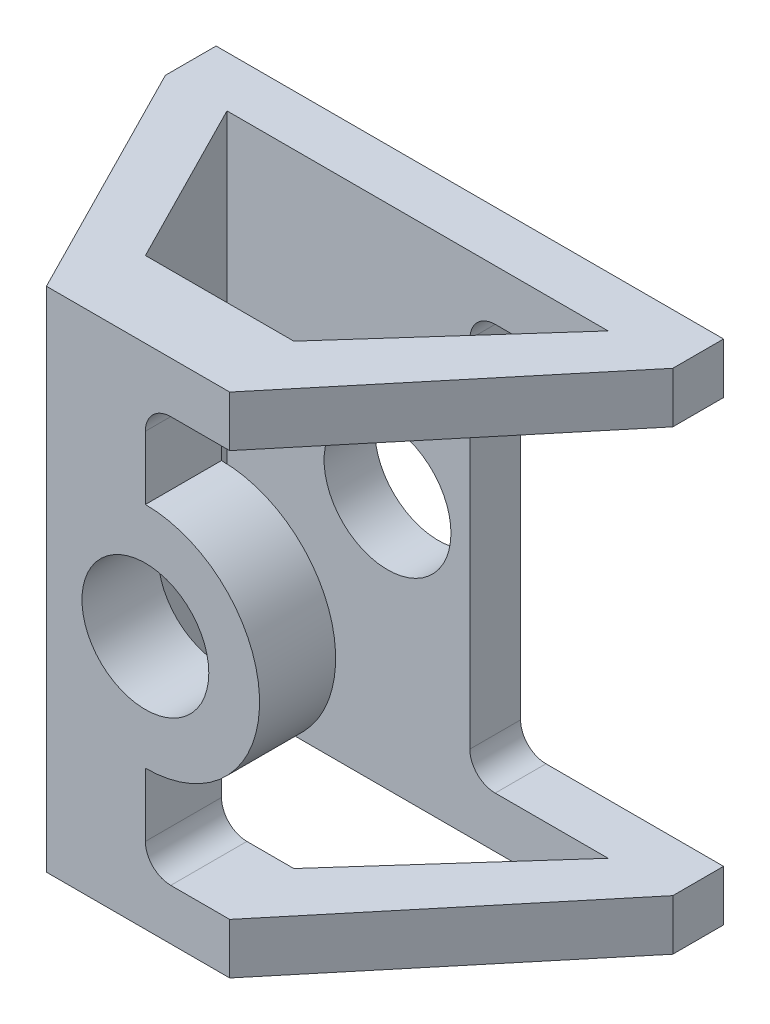
ISO-10303-21;
HEADER;
FILE_DESCRIPTION(('STEP AP214'),'2;1');
FILE_NAME('part.step','',(''),(''),'','','');
FILE_SCHEMA(('AUTOMOTIVE_DESIGN { 1 0 10303 214 1 1 1 1 }'));
ENDSEC;
DATA;
#1=APPLICATION_CONTEXT('core data for automotive mechanical design processes');
#2=APPLICATION_PROTOCOL_DEFINITION('international standard','automotive_design',2000,#1);
#3=PRODUCT_CONTEXT('',#1,'mechanical');
#4=PRODUCT('Part','Part','',(#3));
#5=PRODUCT_RELATED_PRODUCT_CATEGORY('part','',(#4));
#6=PRODUCT_DEFINITION_FORMATION('','',#4);
#7=PRODUCT_DEFINITION_CONTEXT('part definition',#1,'design');
#8=PRODUCT_DEFINITION('design','',#6,#7);
#9=PRODUCT_DEFINITION_SHAPE('','',#8);
#10=(LENGTH_UNIT() NAMED_UNIT(*) SI_UNIT(.MILLI.,.METRE.));
#11=(NAMED_UNIT(*) PLANE_ANGLE_UNIT() SI_UNIT($,.RADIAN.));
#12=(NAMED_UNIT(*) SI_UNIT($,.STERADIAN.) SOLID_ANGLE_UNIT());
#13=UNCERTAINTY_MEASURE_WITH_UNIT(LENGTH_MEASURE(1.E-05),#10,'distance_accuracy_value','');
#14=(GEOMETRIC_REPRESENTATION_CONTEXT(3) GLOBAL_UNCERTAINTY_ASSIGNED_CONTEXT((#13)) GLOBAL_UNIT_ASSIGNED_CONTEXT((#10,
#11,#12)) REPRESENTATION_CONTEXT('',''));
#15=CARTESIAN_POINT('',(0.,0.,0.));
#16=DIRECTION('',(0.,0.,1.));
#17=DIRECTION('',(1.,0.,0.));
#18=AXIS2_PLACEMENT_3D('',#15,#16,#17);
#19=CARTESIAN_POINT('',(87.5566045627291,30.0000000000001,85.4393013950617));
#20=DIRECTION('',(1.,0.,0.));
#21=DIRECTION('',(0.,0.,-1.));
#22=AXIS2_PLACEMENT_3D('',#19,#20,#21);
#23=PLANE('',#22);
#24=DIRECTION('',(0.,0.,1.));
#25=VECTOR('',#24,1.);
#26=CARTESIAN_POINT('',(87.5566045627291,145.,85.4393013950617));
#27=LINE('',#26,#25);
#28=CARTESIAN_POINT('',(87.5566045627291,145.,85.4393013950617));
#29=VERTEX_POINT('',#28);
#30=CARTESIAN_POINT('',(87.5566045627291,145.,115.439301395062));
#31=VERTEX_POINT('',#30);
#32=EDGE_CURVE('E220',#29,#31,#27,.T.);
#33=ORIENTED_EDGE('',*,*,#32,.F.);
#34=DIRECTION('',(0.,1.,0.));
#35=VECTOR('',#34,1.);
#36=CARTESIAN_POINT('',(87.5566045627291,30.0000000000001,85.4393013950617));
#37=LINE('',#36,#35);
#38=CARTESIAN_POINT('',(87.5566045627291,170.,85.4393013950617));
#39=VERTEX_POINT('',#38);
#40=EDGE_CURVE('E226',#29,#39,#37,.T.);
#41=ORIENTED_EDGE('',*,*,#40,.T.);
#42=DIRECTION('',(0.,0.,1.));
#43=VECTOR('',#42,1.);
#44=CARTESIAN_POINT('',(87.5566045627291,170.,85.4393013950617));
#45=LINE('',#44,#43);
#46=CARTESIAN_POINT('',(87.5566045627291,170.,115.439301395062));
#47=VERTEX_POINT('',#46);
#48=EDGE_CURVE('E268',#39,#47,#45,.T.);
#49=ORIENTED_EDGE('',*,*,#48,.T.);
#50=DIRECTION('',(0.,1.,0.));
#51=VECTOR('',#50,1.);
#52=CARTESIAN_POINT('',(87.5566045627291,30.0000000000001,115.439301395062));
#53=LINE('',#52,#51);
#54=EDGE_CURVE('E229',#31,#47,#53,.T.);
#55=ORIENTED_EDGE('',*,*,#54,.F.);
#56=EDGE_LOOP('',(#33,#41,#49,#55));
#57=FACE_BOUND('',#56,.T.);
#58=ADVANCED_FACE('F50',(#57),#23,.T.);
#59=CARTESIAN_POINT('',(107.014759016757,200.,95.5723404549719));
#60=DIRECTION('',(0.745856464082351,0.,0.666106699400759));
#61=DIRECTION('',(0.666106699400759,0.,-0.745856464082351));
#62=AXIS2_PLACEMENT_3D('',#59,#60,#61);
#63=PLANE('',#62);
#64=DIRECTION('',(0.,-1.,0.));
#65=VECTOR('',#64,1.);
#66=CARTESIAN_POINT('',(116.064335615118,200.,85.4393013950617));
#67=LINE('',#66,#65);
#68=CARTESIAN_POINT('',(116.064335615118,20.,85.4393013950617));
#69=VERTEX_POINT('',#68);
#70=CARTESIAN_POINT('',(116.064335615118,0.,85.4393013950617));
#71=VERTEX_POINT('',#70);
#72=EDGE_CURVE('E271',#69,#71,#67,.T.);
#73=ORIENTED_EDGE('',*,*,#72,.F.);
#74=DIRECTION('',(0.666106699400759,0.,-0.745856464082351));
#75=VECTOR('',#74,1.);
#76=CARTESIAN_POINT('',(107.014759016757,20.,95.5723404549719));
#77=LINE('',#76,#75);
#78=CARTESIAN_POINT('',(174.50662198316,20.,20.));
#79=VERTEX_POINT('',#78);
#80=EDGE_CURVE('E57',#69,#79,#77,.T.);
#81=ORIENTED_EDGE('',*,*,#80,.T.);
#82=DIRECTION('',(0.,1.,0.));
#83=VECTOR('',#82,1.);
#84=CARTESIAN_POINT('',(174.50662198316,0.,20.));
#85=LINE('',#84,#83);
#86=CARTESIAN_POINT('',(174.50662198316,0.,20.));
#87=VERTEX_POINT('',#86);
#88=EDGE_CURVE('E400',#87,#79,#85,.T.);
#89=ORIENTED_EDGE('',*,*,#88,.F.);
#90=DIRECTION('',(-0.666106699400759,0.,0.745856464082351));
#91=VECTOR('',#90,1.);
#92=CARTESIAN_POINT('',(107.014759016757,0.,95.5723404549719));
#93=LINE('',#92,#91);
#94=EDGE_CURVE('E282',#87,#71,#93,.T.);
#95=ORIENTED_EDGE('',*,*,#94,.T.);
#96=EDGE_LOOP('',(#73,#81,#89,#95));
#97=FACE_BOUND('',#96,.T.);
#98=ADVANCED_FACE('F408',(#97),#63,.F.);
#99=CARTESIAN_POINT('',(11.2035333427631,200.,-5.70043815756806));
#100=DIRECTION('',(0.891265334485345,0.,-0.453482197605072));
#101=DIRECTION('',(-0.453482197605072,0.,-0.891265334485345));
#102=AXIS2_PLACEMENT_3D('',#99,#100,#101);
#103=PLANE('',#102);
#104=DIRECTION('',(0.453482197605073,0.,0.891265334485345));
#105=VECTOR('',#104,1.);
#106=CARTESIAN_POINT('',(11.2035333427631,200.,-5.70043815756806));
#107=LINE('',#106,#105);
#108=CARTESIAN_POINT('',(24.2801006949952,200.,20.));
#109=VERTEX_POINT('',#108);
#110=CARTESIAN_POINT('',(57.5760868151209,200.,85.4393013950617));
#111=VERTEX_POINT('',#110);
#112=EDGE_CURVE('E73',#109,#111,#107,.T.);
#113=ORIENTED_EDGE('',*,*,#112,.T.);
#114=DIRECTION('',(0.,-1.,0.));
#115=VECTOR('',#114,1.);
#116=CARTESIAN_POINT('',(57.5760868151209,200.,85.4393013950617));
#117=LINE('',#116,#115);
#118=CARTESIAN_POINT('',(57.5760868151209,0.,85.4393013950617));
#119=VERTEX_POINT('',#118);
#120=EDGE_CURVE('E264',#111,#119,#117,.T.);
#121=ORIENTED_EDGE('',*,*,#120,.T.);
#122=DIRECTION('',(0.453482197605073,0.,0.891265334485345));
#123=VECTOR('',#122,1.);
#124=CARTESIAN_POINT('',(11.2035333427631,0.,-5.70043815756806));
#125=LINE('',#124,#123);
#126=CARTESIAN_POINT('',(24.2801006949951,0.,20.));
#127=VERTEX_POINT('',#126);
#128=EDGE_CURVE('E290',#127,#119,#125,.T.);
#129=ORIENTED_EDGE('',*,*,#128,.F.);
#130=DIRECTION('',(0.,-1.,0.));
#131=VECTOR('',#130,1.);
#132=CARTESIAN_POINT('',(24.2801006949951,200.,20.));
#133=LINE('',#132,#131);
#134=EDGE_CURVE('E311',#109,#127,#133,.T.);
#135=ORIENTED_EDGE('',*,*,#134,.F.);
#136=EDGE_LOOP('',(#113,#121,#129,#135));
#137=FACE_BOUND('',#136,.T.);
#138=ADVANCED_FACE('F442',(#137),#103,.T.);
#139=DIRECTION('',(0.,-1.,0.));
#140=VECTOR('',#139,1.);
#141=CARTESIAN_POINT('',(116.064335615118,200.,85.4393013950617));
#142=LINE('',#141,#140);
#143=CARTESIAN_POINT('',(116.064335615118,200.,85.4393013950617));
#144=VERTEX_POINT('',#143);
#145=CARTESIAN_POINT('',(116.064335615118,180.,85.4393013950617));
#146=VERTEX_POINT('',#145);
#147=EDGE_CURVE('E11',#144,#146,#142,.T.);
#148=ORIENTED_EDGE('',*,*,#147,.F.);
#149=DIRECTION('',(-0.666106699400759,0.,0.745856464082351));
#150=VECTOR('',#149,1.);
#151=CARTESIAN_POINT('',(107.014759016757,200.,95.5723404549719));
#152=LINE('',#151,#150);
#153=CARTESIAN_POINT('',(174.50662198316,200.,20.));
#154=VERTEX_POINT('',#153);
#155=EDGE_CURVE('E284',#154,#144,#152,.T.);
#156=ORIENTED_EDGE('',*,*,#155,.F.);
#157=DIRECTION('',(0.,-1.,0.));
#158=VECTOR('',#157,1.);
#159=CARTESIAN_POINT('',(174.50662198316,200.,20.));
#160=LINE('',#159,#158);
#161=CARTESIAN_POINT('',(174.50662198316,180.,20.));
#162=VERTEX_POINT('',#161);
#163=EDGE_CURVE('E296',#154,#162,#160,.T.);
#164=ORIENTED_EDGE('',*,*,#163,.T.);
#165=DIRECTION('',(-0.666106699400759,0.,0.745856464082351));
#166=VECTOR('',#165,1.);
#167=CARTESIAN_POINT('',(107.014759016757,180.,95.5723404549719));
#168=LINE('',#167,#166);
#169=EDGE_CURVE('E405',#162,#146,#168,.T.);
#170=ORIENTED_EDGE('',*,*,#169,.T.);
#171=EDGE_LOOP('',(#148,#156,#164,#170));
#172=FACE_BOUND('',#171,.T.);
#173=ADVANCED_FACE('F437',(#172),#63,.F.);
#174=CARTESIAN_POINT('',(128.259685240505,200.,106.443715140529));
#175=DIRECTION('',(0.769516093689913,0.,0.638627419981492));
#176=DIRECTION('',(0.638627419981492,0.,-0.769516093689913));
#177=AXIS2_PLACEMENT_3D('',#174,#175,#176);
#178=PLANE('',#177);
#179=DIRECTION('',(0.638627419981492,0.,-0.769516093689913));
#180=VECTOR('',#179,1.);
#181=CARTESIAN_POINT('',(200.,20.,20.));
#182=LINE('',#181,#180);
#183=CARTESIAN_POINT('',(120.794177906661,20.,115.439301395062));
#184=VERTEX_POINT('',#183);
#185=CARTESIAN_POINT('',(200.,20.,20.));
#186=VERTEX_POINT('',#185);
#187=EDGE_CURVE('E285',#184,#186,#182,.T.);
#188=ORIENTED_EDGE('',*,*,#187,.F.);
#189=DIRECTION('',(0.,-1.,0.));
#190=VECTOR('',#189,1.);
#191=CARTESIAN_POINT('',(120.794177906661,200.,115.439301395062));
#192=LINE('',#191,#190);
#193=CARTESIAN_POINT('',(120.794177906661,0.,115.439301395062));
#194=VERTEX_POINT('',#193);
#195=EDGE_CURVE('E324',#184,#194,#192,.T.);
#196=ORIENTED_EDGE('',*,*,#195,.T.);
#197=DIRECTION('',(-0.638627419981492,0.,0.769516093689913));
#198=VECTOR('',#197,1.);
#199=CARTESIAN_POINT('',(128.259685240505,0.,106.443715140529));
#200=LINE('',#199,#198);
#201=CARTESIAN_POINT('',(200.,0.,20.));
#202=VERTEX_POINT('',#201);
#203=EDGE_CURVE('E301',#202,#194,#200,.T.);
#204=ORIENTED_EDGE('',*,*,#203,.F.);
#205=DIRECTION('',(0.,1.,0.));
#206=VECTOR('',#205,1.);
#207=CARTESIAN_POINT('',(200.,0.,20.));
#208=LINE('',#207,#206);
#209=EDGE_CURVE('E345',#202,#186,#208,.T.);
#210=ORIENTED_EDGE('',*,*,#209,.T.);
#211=EDGE_LOOP('',(#188,#196,#204,#210));
#212=FACE_BOUND('',#211,.T.);
#213=ADVANCED_FACE('F506',(#212),#178,.T.);
#214=CARTESIAN_POINT('',(0.,0.,20.));
#215=DIRECTION('',(0.,0.,1.));
#216=DIRECTION('',(1.,0.,0.));
#217=AXIS2_PLACEMENT_3D('',#214,#215,#216);
#218=PLANE('',#217);
#219=CARTESIAN_POINT('',(87.5566045627291,100.,20.));
#220=DIRECTION('',(0.,0.,1.));
#221=DIRECTION('',(1.,0.,0.));
#222=AXIS2_PLACEMENT_3D('',#219,#220,#221);
#223=CIRCLE('',#222,25.);
#224=CARTESIAN_POINT('',(112.556604562729,100.,20.));
#225=VERTEX_POINT('',#224);
#226=EDGE_CURVE('E451',#225,#225,#223,.T.);
#227=ORIENTED_EDGE('',*,*,#226,.F.);
#228=EDGE_LOOP('',(#227));
#229=FACE_BOUND('',#228,.T.);
#230=ORIENTED_EDGE('',*,*,#134,.T.);
#231=DIRECTION('',(1.,0.,0.));
#232=VECTOR('',#231,1.);
#233=CARTESIAN_POINT('',(0.,0.,20.));
#234=LINE('',#233,#232);
#235=EDGE_CURVE('E344',#127,#87,#234,.T.);
#236=ORIENTED_EDGE('',*,*,#235,.T.);
#237=ORIENTED_EDGE('',*,*,#88,.T.);
#238=DIRECTION('',(-1.,0.,0.));
#239=VECTOR('',#238,1.);
#240=CARTESIAN_POINT('',(0.,20.,20.));
#241=LINE('',#240,#239);
#242=CARTESIAN_POINT('',(130.,20.,20.));
#243=VERTEX_POINT('',#242);
#244=EDGE_CURVE('E346',#79,#243,#241,.T.);
#245=ORIENTED_EDGE('',*,*,#244,.T.);
#246=CARTESIAN_POINT('',(130.,30.,20.));
#247=DIRECTION('',(0.,0.,1.));
#248=DIRECTION('',(1.,0.,0.));
#249=AXIS2_PLACEMENT_3D('',#246,#247,#248);
#250=CIRCLE('',#249,10.);
#251=CARTESIAN_POINT('',(120.,30.0000000000001,20.));
#252=VERTEX_POINT('',#251);
#253=EDGE_CURVE('E348',#243,#252,#250,.F.);
#254=ORIENTED_EDGE('',*,*,#253,.T.);
#255=DIRECTION('',(0.,1.,0.));
#256=VECTOR('',#255,1.);
#257=CARTESIAN_POINT('',(120.,0.,20.));
#258=LINE('',#257,#256);
#259=CARTESIAN_POINT('',(120.,170.,20.));
#260=VERTEX_POINT('',#259);
#261=EDGE_CURVE('E323',#252,#260,#258,.T.);
#262=ORIENTED_EDGE('',*,*,#261,.T.);
#263=CARTESIAN_POINT('',(130.,170.,20.));
#264=DIRECTION('',(0.,0.,1.));
#265=DIRECTION('',(1.,0.,0.));
#266=AXIS2_PLACEMENT_3D('',#263,#264,#265);
#267=CIRCLE('',#266,10.);
#268=CARTESIAN_POINT('',(130.,180.,20.));
#269=VERTEX_POINT('',#268);
#270=EDGE_CURVE('E330',#260,#269,#267,.F.);
#271=ORIENTED_EDGE('',*,*,#270,.T.);
#272=DIRECTION('',(-1.,0.,0.));
#273=VECTOR('',#272,1.);
#274=CARTESIAN_POINT('',(0.,180.,20.));
#275=LINE('',#274,#273);
#276=EDGE_CURVE('E333',#162,#269,#275,.T.);
#277=ORIENTED_EDGE('',*,*,#276,.F.);
#278=ORIENTED_EDGE('',*,*,#163,.F.);
#279=DIRECTION('',(-1.,0.,0.));
#280=VECTOR('',#279,1.);
#281=CARTESIAN_POINT('',(0.,200.,20.));
#282=LINE('',#281,#280);
#283=EDGE_CURVE('E337',#154,#109,#282,.T.);
#284=ORIENTED_EDGE('',*,*,#283,.T.);
#285=EDGE_LOOP('',(#230,#236,#237,#245,#254,#262,#271,#277,#278,#284));
#286=FACE_BOUND('',#285,.T.);
#287=ADVANCED_FACE('F412',(#229,#286),#218,.T.);
#288=CARTESIAN_POINT('',(120.,0.,20.));
#289=DIRECTION('',(-1.,0.,0.));
#290=DIRECTION('',(0.,0.,1.));
#291=AXIS2_PLACEMENT_3D('',#288,#289,#290);
#292=PLANE('',#291);
#293=DIRECTION('',(0.,1.,0.));
#294=VECTOR('',#293,1.);
#295=CARTESIAN_POINT('',(120.,0.,0.));
#296=LINE('',#295,#294);
#297=CARTESIAN_POINT('',(120.,30.0000000000001,0.));
#298=VERTEX_POINT('',#297);
#299=CARTESIAN_POINT('',(120.,170.,0.));
#300=VERTEX_POINT('',#299);
#301=EDGE_CURVE('E313',#298,#300,#296,.T.);
#302=ORIENTED_EDGE('',*,*,#301,.T.);
#303=DIRECTION('',(0.,0.,-1.));
#304=VECTOR('',#303,1.);
#305=CARTESIAN_POINT('',(120.,170.,20.));
#306=LINE('',#305,#304);
#307=EDGE_CURVE('E398',#260,#300,#306,.T.);
#308=ORIENTED_EDGE('',*,*,#307,.F.);
#309=ORIENTED_EDGE('',*,*,#261,.F.);
#310=DIRECTION('',(0.,0.,-1.));
#311=VECTOR('',#310,1.);
#312=CARTESIAN_POINT('',(120.,30.0000000000001,20.));
#313=LINE('',#312,#311);
#314=EDGE_CURVE('E349',#252,#298,#313,.T.);
#315=ORIENTED_EDGE('',*,*,#314,.T.);
#316=EDGE_LOOP('',(#302,#308,#309,#315));
#317=FACE_BOUND('',#316,.T.);
#318=ADVANCED_FACE('F47',(#317),#292,.F.);
#319=CARTESIAN_POINT('',(130.,170.,20.));
#320=DIRECTION('',(0.,0.,-1.));
#321=DIRECTION('',(-1.,0.,0.));
#322=AXIS2_PLACEMENT_3D('',#319,#320,#321);
#323=CYLINDRICAL_SURFACE('',#322,10.);
#324=CARTESIAN_POINT('',(130.,170.,0.));
#325=DIRECTION('',(0.,0.,1.));
#326=DIRECTION('',(1.,0.,0.));
#327=AXIS2_PLACEMENT_3D('',#324,#325,#326);
#328=CIRCLE('',#327,10.);
#329=CARTESIAN_POINT('',(130.,180.,0.));
#330=VERTEX_POINT('',#329);
#331=EDGE_CURVE('E352',#300,#330,#328,.F.);
#332=ORIENTED_EDGE('',*,*,#331,.T.);
#333=DIRECTION('',(0.,0.,-1.));
#334=VECTOR('',#333,1.);
#335=CARTESIAN_POINT('',(130.,180.,20.));
#336=LINE('',#335,#334);
#337=EDGE_CURVE('E392',#269,#330,#336,.T.);
#338=ORIENTED_EDGE('',*,*,#337,.F.);
#339=ORIENTED_EDGE('',*,*,#270,.F.);
#340=ORIENTED_EDGE('',*,*,#307,.T.);
#341=EDGE_LOOP('',(#332,#338,#339,#340));
#342=FACE_BOUND('',#341,.T.);
#343=ADVANCED_FACE('F427',(#342),#323,.F.);
#344=CARTESIAN_POINT('',(0.,180.,20.));
#345=DIRECTION('',(0.,-1.,0.));
#346=DIRECTION('',(0.,0.,-1.));
#347=AXIS2_PLACEMENT_3D('',#344,#345,#346);
#348=PLANE('',#347);
#349=DIRECTION('',(-0.638627419981492,0.,0.769516093689913));
#350=VECTOR('',#349,1.);
#351=CARTESIAN_POINT('',(200.,180.,20.));
#352=LINE('',#351,#350);
#353=CARTESIAN_POINT('',(200.,180.,20.));
#354=VERTEX_POINT('',#353);
#355=CARTESIAN_POINT('',(120.794177906661,180.,115.439301395062));
#356=VERTEX_POINT('',#355);
#357=EDGE_CURVE('E278',#354,#356,#352,.T.);
#358=ORIENTED_EDGE('',*,*,#357,.T.);
#359=DIRECTION('',(-1.,0.,0.));
#360=VECTOR('',#359,1.);
#361=CARTESIAN_POINT('',(120.794177906661,180.,115.439301395062));
#362=LINE('',#361,#360);
#363=CARTESIAN_POINT('',(97.5566045627291,180.,115.439301395062));
#364=VERTEX_POINT('',#363);
#365=EDGE_CURVE('E273',#356,#364,#362,.T.);
#366=ORIENTED_EDGE('',*,*,#365,.T.);
#367=DIRECTION('',(0.,0.,1.));
#368=VECTOR('',#367,1.);
#369=CARTESIAN_POINT('',(97.5566045627291,180.,85.4393013950617));
#370=LINE('',#369,#368);
#371=CARTESIAN_POINT('',(97.5566045627291,180.,85.4393013950617));
#372=VERTEX_POINT('',#371);
#373=EDGE_CURVE('E265',#372,#364,#370,.T.);
#374=ORIENTED_EDGE('',*,*,#373,.F.);
#375=DIRECTION('',(1.,0.,0.));
#376=VECTOR('',#375,1.);
#377=CARTESIAN_POINT('',(120.794177906661,180.,85.4393013950617));
#378=LINE('',#377,#376);
#379=EDGE_CURVE('E246',#372,#146,#378,.T.);
#380=ORIENTED_EDGE('',*,*,#379,.T.);
#381=ORIENTED_EDGE('',*,*,#169,.F.);
#382=ORIENTED_EDGE('',*,*,#276,.T.);
#383=ORIENTED_EDGE('',*,*,#337,.T.);
#384=DIRECTION('',(-1.,0.,0.));
#385=VECTOR('',#384,1.);
#386=CARTESIAN_POINT('',(0.,180.,0.));
#387=LINE('',#386,#385);
#388=CARTESIAN_POINT('',(200.,180.,0.));
#389=VERTEX_POINT('',#388);
#390=EDGE_CURVE('E358',#389,#330,#387,.T.);
#391=ORIENTED_EDGE('',*,*,#390,.F.);
#392=DIRECTION('',(0.,0.,-1.));
#393=VECTOR('',#392,1.);
#394=CARTESIAN_POINT('',(200.,180.,20.));
#395=LINE('',#394,#393);
#396=EDGE_CURVE('E395',#354,#389,#395,.T.);
#397=ORIENTED_EDGE('',*,*,#396,.F.);
#398=EDGE_LOOP('',(#358,#366,#374,#380,#381,#382,#383,#391,#397));
#399=FACE_BOUND('',#398,.T.);
#400=ADVANCED_FACE('F433',(#399),#348,.T.);
#401=CARTESIAN_POINT('',(200.,0.,20.));
#402=DIRECTION('',(1.,0.,0.));
#403=DIRECTION('',(0.,0.,-1.));
#404=AXIS2_PLACEMENT_3D('',#401,#402,#403);
#405=PLANE('',#404);
#406=DIRECTION('',(0.,-1.,0.));
#407=VECTOR('',#406,1.);
#408=CARTESIAN_POINT('',(200.,0.,0.));
#409=LINE('',#408,#407);
#410=CARTESIAN_POINT('',(200.,200.,0.));
#411=VERTEX_POINT('',#410);
#412=EDGE_CURVE('E360',#411,#389,#409,.T.);
#413=ORIENTED_EDGE('',*,*,#412,.F.);
#414=DIRECTION('',(0.,0.,-1.));
#415=VECTOR('',#414,1.);
#416=CARTESIAN_POINT('',(200.,200.,20.));
#417=LINE('',#416,#415);
#418=CARTESIAN_POINT('',(200.,200.,20.));
#419=VERTEX_POINT('',#418);
#420=EDGE_CURVE('E387',#419,#411,#417,.T.);
#421=ORIENTED_EDGE('',*,*,#420,.F.);
#422=DIRECTION('',(0.,-1.,0.));
#423=VECTOR('',#422,1.);
#424=CARTESIAN_POINT('',(200.,0.,20.));
#425=LINE('',#424,#423);
#426=EDGE_CURVE('E332',#419,#354,#425,.T.);
#427=ORIENTED_EDGE('',*,*,#426,.T.);
#428=ORIENTED_EDGE('',*,*,#396,.T.);
#429=EDGE_LOOP('',(#413,#421,#427,#428));
#430=FACE_BOUND('',#429,.T.);
#431=ADVANCED_FACE('F525',(#430),#405,.T.);
#432=CARTESIAN_POINT('',(0.,200.,20.));
#433=DIRECTION('',(0.,-1.,0.));
#434=DIRECTION('',(0.,0.,-1.));
#435=AXIS2_PLACEMENT_3D('',#432,#433,#434);
#436=PLANE('',#435);
#437=DIRECTION('',(-1.,0.,0.));
#438=VECTOR('',#437,1.);
#439=CARTESIAN_POINT('',(0.,200.,115.439301395062));
#440=LINE('',#439,#438);
#441=CARTESIAN_POINT('',(120.794177906661,200.,115.439301395062));
#442=VERTEX_POINT('',#441);
#443=CARTESIAN_POINT('',(48.5602013899903,200.,115.439301395062));
#444=VERTEX_POINT('',#443);
#445=EDGE_CURVE('E292',#442,#444,#440,.T.);
#446=ORIENTED_EDGE('',*,*,#445,.F.);
#447=DIRECTION('',(-0.638627419981492,0.,0.769516093689913));
#448=VECTOR('',#447,1.);
#449=CARTESIAN_POINT('',(128.259685240505,200.,106.443715140529));
#450=LINE('',#449,#448);
#451=EDGE_CURVE('E287',#419,#442,#450,.T.);
#452=ORIENTED_EDGE('',*,*,#451,.F.);
#453=ORIENTED_EDGE('',*,*,#420,.T.);
#454=DIRECTION('',(-1.,0.,0.));
#455=VECTOR('',#454,1.);
#456=CARTESIAN_POINT('',(0.,200.,0.));
#457=LINE('',#456,#455);
#458=CARTESIAN_POINT('',(0.,200.,0.));
#459=VERTEX_POINT('',#458);
#460=EDGE_CURVE('E365',#411,#459,#457,.T.);
#461=ORIENTED_EDGE('',*,*,#460,.T.);
#462=DIRECTION('',(0.,0.,-1.));
#463=VECTOR('',#462,1.);
#464=CARTESIAN_POINT('',(0.,200.,20.));
#465=LINE('',#464,#463);
#466=CARTESIAN_POINT('',(0.,200.,20.));
#467=VERTEX_POINT('',#466);
#468=EDGE_CURVE('E390',#467,#459,#465,.T.);
#469=ORIENTED_EDGE('',*,*,#468,.F.);
#470=DIRECTION('',(-0.453482197605073,0.,-0.891265334485345));
#471=VECTOR('',#470,1.);
#472=CARTESIAN_POINT('',(-8.08345925063269,200.,4.11292207089452));
#473=LINE('',#472,#471);
#474=EDGE_CURVE('E295',#444,#467,#473,.T.);
#475=ORIENTED_EDGE('',*,*,#474,.F.);
#476=EDGE_LOOP('',(#446,#452,#453,#461,#469,#475));
#477=FACE_BOUND('',#476,.T.);
#478=ORIENTED_EDGE('',*,*,#155,.T.);
#479=DIRECTION('',(-1.,0.,0.));
#480=VECTOR('',#479,1.);
#481=CARTESIAN_POINT('',(48.5602013899903,200.,85.4393013950617));
#482=LINE('',#481,#480);
#483=EDGE_CURVE('E248',#144,#111,#482,.T.);
#484=ORIENTED_EDGE('',*,*,#483,.T.);
#485=ORIENTED_EDGE('',*,*,#112,.F.);
#486=ORIENTED_EDGE('',*,*,#283,.F.);
#487=EDGE_LOOP('',(#478,#484,#485,#486));
#488=FACE_BOUND('',#487,.T.);
#489=ADVANCED_FACE('F441',(#477,#488),#436,.F.);
#490=CARTESIAN_POINT('',(0.,0.,20.));
#491=DIRECTION('',(-1.,0.,0.));
#492=DIRECTION('',(0.,0.,1.));
#493=AXIS2_PLACEMENT_3D('',#490,#491,#492);
#494=PLANE('',#493);
#495=DIRECTION('',(0.,1.,0.));
#496=VECTOR('',#495,1.);
#497=CARTESIAN_POINT('',(0.,0.,0.));
#498=LINE('',#497,#496);
#499=CARTESIAN_POINT('',(0.,0.,0.));
#500=VERTEX_POINT('',#499);
#501=EDGE_CURVE('E362',#500,#459,#498,.T.);
#502=ORIENTED_EDGE('',*,*,#501,.F.);
#503=DIRECTION('',(0.,0.,-1.));
#504=VECTOR('',#503,1.);
#505=CARTESIAN_POINT('',(0.,0.,20.));
#506=LINE('',#505,#504);
#507=CARTESIAN_POINT('',(0.,0.,20.));
#508=VERTEX_POINT('',#507);
#509=EDGE_CURVE('E389',#508,#500,#506,.T.);
#510=ORIENTED_EDGE('',*,*,#509,.F.);
#511=DIRECTION('',(0.,1.,0.));
#512=VECTOR('',#511,1.);
#513=CARTESIAN_POINT('',(0.,0.,20.));
#514=LINE('',#513,#512);
#515=EDGE_CURVE('E336',#508,#467,#514,.T.);
#516=ORIENTED_EDGE('',*,*,#515,.T.);
#517=ORIENTED_EDGE('',*,*,#468,.T.);
#518=EDGE_LOOP('',(#502,#510,#516,#517));
#519=FACE_BOUND('',#518,.T.);
#520=ADVANCED_FACE('F534',(#519),#494,.T.);
#521=CARTESIAN_POINT('',(0.,0.,20.));
#522=DIRECTION('',(0.,1.,0.));
#523=DIRECTION('',(0.,0.,1.));
#524=AXIS2_PLACEMENT_3D('',#521,#522,#523);
#525=PLANE('',#524);
#526=DIRECTION('',(1.,0.,0.));
#527=VECTOR('',#526,1.);
#528=CARTESIAN_POINT('',(120.794177906661,0.,85.4393013950617));
#529=LINE('',#528,#527);
#530=EDGE_CURVE('E261',#119,#71,#529,.T.);
#531=ORIENTED_EDGE('',*,*,#530,.T.);
#532=ORIENTED_EDGE('',*,*,#94,.F.);
#533=ORIENTED_EDGE('',*,*,#235,.F.);
#534=ORIENTED_EDGE('',*,*,#128,.T.);
#535=EDGE_LOOP('',(#531,#532,#533,#534));
#536=FACE_BOUND('',#535,.T.);
#537=DIRECTION('',(-1.,0.,0.));
#538=VECTOR('',#537,1.);
#539=CARTESIAN_POINT('',(0.,0.,115.439301395062));
#540=LINE('',#539,#538);
#541=CARTESIAN_POINT('',(48.5602013899903,0.,115.439301395062));
#542=VERTEX_POINT('',#541);
#543=EDGE_CURVE('E302',#194,#542,#540,.T.);
#544=ORIENTED_EDGE('',*,*,#543,.T.);
#545=DIRECTION('',(-0.453482197605073,0.,-0.891265334485345));
#546=VECTOR('',#545,1.);
#547=CARTESIAN_POINT('',(-8.08345925063269,0.,4.11292207089452));
#548=LINE('',#547,#546);
#549=EDGE_CURVE('E306',#542,#508,#548,.T.);
#550=ORIENTED_EDGE('',*,*,#549,.T.);
#551=ORIENTED_EDGE('',*,*,#509,.T.);
#552=DIRECTION('',(1.,0.,0.));
#553=VECTOR('',#552,1.);
#554=CARTESIAN_POINT('',(0.,0.,0.));
#555=LINE('',#554,#553);
#556=CARTESIAN_POINT('',(200.,0.,0.));
#557=VERTEX_POINT('',#556);
#558=EDGE_CURVE('E368',#500,#557,#555,.T.);
#559=ORIENTED_EDGE('',*,*,#558,.T.);
#560=DIRECTION('',(0.,0.,-1.));
#561=VECTOR('',#560,1.);
#562=CARTESIAN_POINT('',(200.,0.,20.));
#563=LINE('',#562,#561);
#564=EDGE_CURVE('E384',#202,#557,#563,.T.);
#565=ORIENTED_EDGE('',*,*,#564,.F.);
#566=ORIENTED_EDGE('',*,*,#203,.T.);
#567=EDGE_LOOP('',(#544,#550,#551,#559,#565,#566));
#568=FACE_BOUND('',#567,.T.);
#569=ADVANCED_FACE('F450',(#536,#568),#525,.F.);
#570=CARTESIAN_POINT('',(200.,0.,20.));
#571=DIRECTION('',(-1.,0.,0.));
#572=DIRECTION('',(0.,0.,1.));
#573=AXIS2_PLACEMENT_3D('',#570,#571,#572);
#574=PLANE('',#573);
#575=DIRECTION('',(0.,1.,0.));
#576=VECTOR('',#575,1.);
#577=CARTESIAN_POINT('',(200.,0.,0.));
#578=LINE('',#577,#576);
#579=CARTESIAN_POINT('',(200.,20.,0.));
#580=VERTEX_POINT('',#579);
#581=EDGE_CURVE('E369',#557,#580,#578,.T.);
#582=ORIENTED_EDGE('',*,*,#581,.T.);
#583=DIRECTION('',(0.,0.,-1.));
#584=VECTOR('',#583,1.);
#585=CARTESIAN_POINT('',(200.,20.,20.));
#586=LINE('',#585,#584);
#587=EDGE_CURVE('E379',#186,#580,#586,.T.);
#588=ORIENTED_EDGE('',*,*,#587,.F.);
#589=ORIENTED_EDGE('',*,*,#209,.F.);
#590=ORIENTED_EDGE('',*,*,#564,.T.);
#591=EDGE_LOOP('',(#582,#588,#589,#590));
#592=FACE_BOUND('',#591,.T.);
#593=ADVANCED_FACE('F513',(#592),#574,.F.);
#594=CARTESIAN_POINT('',(0.,20.,20.));
#595=DIRECTION('',(0.,-1.,0.));
#596=DIRECTION('',(0.,0.,-1.));
#597=AXIS2_PLACEMENT_3D('',#594,#595,#596);
#598=PLANE('',#597);
#599=ORIENTED_EDGE('',*,*,#80,.F.);
#600=DIRECTION('',(-1.,0.,0.));
#601=VECTOR('',#600,1.);
#602=CARTESIAN_POINT('',(120.794177906661,20.,85.4393013950617));
#603=LINE('',#602,#601);
#604=CARTESIAN_POINT('',(97.5566045627291,20.,85.4393013950617));
#605=VERTEX_POINT('',#604);
#606=EDGE_CURVE('E241',#69,#605,#603,.T.);
#607=ORIENTED_EDGE('',*,*,#606,.T.);
#608=DIRECTION('',(0.,0.,1.));
#609=VECTOR('',#608,1.);
#610=CARTESIAN_POINT('',(97.5566045627291,20.,85.4393013950617));
#611=LINE('',#610,#609);
#612=CARTESIAN_POINT('',(97.5566045627291,20.,115.439301395062));
#613=VERTEX_POINT('',#612);
#614=EDGE_CURVE('E255',#605,#613,#611,.T.);
#615=ORIENTED_EDGE('',*,*,#614,.T.);
#616=DIRECTION('',(1.,0.,0.));
#617=VECTOR('',#616,1.);
#618=CARTESIAN_POINT('',(77.428259439369,20.,115.439301395062));
#619=LINE('',#618,#617);
#620=EDGE_CURVE('E276',#613,#184,#619,.T.);
#621=ORIENTED_EDGE('',*,*,#620,.T.);
#622=ORIENTED_EDGE('',*,*,#187,.T.);
#623=ORIENTED_EDGE('',*,*,#587,.T.);
#624=DIRECTION('',(-1.,0.,0.));
#625=VECTOR('',#624,1.);
#626=CARTESIAN_POINT('',(0.,20.,0.));
#627=LINE('',#626,#625);
#628=CARTESIAN_POINT('',(130.,20.,0.));
#629=VERTEX_POINT('',#628);
#630=EDGE_CURVE('E375',#580,#629,#627,.T.);
#631=ORIENTED_EDGE('',*,*,#630,.T.);
#632=DIRECTION('',(0.,0.,-1.));
#633=VECTOR('',#632,1.);
#634=CARTESIAN_POINT('',(130.,20.,20.));
#635=LINE('',#634,#633);
#636=EDGE_CURVE('E380',#243,#629,#635,.T.);
#637=ORIENTED_EDGE('',*,*,#636,.F.);
#638=ORIENTED_EDGE('',*,*,#244,.F.);
#639=EDGE_LOOP('',(#599,#607,#615,#621,#622,#623,#631,#637,#638));
#640=FACE_BOUND('',#639,.T.);
#641=ADVANCED_FACE('F418',(#640),#598,.F.);
#642=CARTESIAN_POINT('',(130.,30.,20.));
#643=DIRECTION('',(0.,0.,-1.));
#644=DIRECTION('',(-1.,0.,0.));
#645=AXIS2_PLACEMENT_3D('',#642,#643,#644);
#646=CYLINDRICAL_SURFACE('',#645,10.);
#647=CARTESIAN_POINT('',(130.,30.,0.));
#648=DIRECTION('',(0.,0.,1.));
#649=DIRECTION('',(1.,0.,0.));
#650=AXIS2_PLACEMENT_3D('',#647,#648,#649);
#651=CIRCLE('',#650,10.);
#652=EDGE_CURVE('E328',#629,#298,#651,.F.);
#653=ORIENTED_EDGE('',*,*,#652,.T.);
#654=ORIENTED_EDGE('',*,*,#314,.F.);
#655=ORIENTED_EDGE('',*,*,#253,.F.);
#656=ORIENTED_EDGE('',*,*,#636,.T.);
#657=EDGE_LOOP('',(#653,#654,#655,#656));
#658=FACE_BOUND('',#657,.T.);
#659=ADVANCED_FACE('F422',(#658),#646,.F.);
#660=CARTESIAN_POINT('',(0.,0.,0.));
#661=DIRECTION('',(0.,0.,1.));
#662=DIRECTION('',(1.,0.,0.));
#663=AXIS2_PLACEMENT_3D('',#660,#661,#662);
#664=PLANE('',#663);
#665=CARTESIAN_POINT('',(87.5566045627291,100.,0.));
#666=DIRECTION('',(0.,0.,1.));
#667=DIRECTION('',(1.,0.,0.));
#668=AXIS2_PLACEMENT_3D('',#665,#666,#667);
#669=CIRCLE('',#668,25.);
#670=CARTESIAN_POINT('',(112.556604562729,100.,0.));
#671=VERTEX_POINT('',#670);
#672=EDGE_CURVE('E456',#671,#671,#669,.T.);
#673=ORIENTED_EDGE('',*,*,#672,.T.);
#674=EDGE_LOOP('',(#673));
#675=FACE_BOUND('',#674,.T.);
#676=ORIENTED_EDGE('',*,*,#301,.F.);
#677=ORIENTED_EDGE('',*,*,#652,.F.);
#678=ORIENTED_EDGE('',*,*,#630,.F.);
#679=ORIENTED_EDGE('',*,*,#581,.F.);
#680=ORIENTED_EDGE('',*,*,#558,.F.);
#681=ORIENTED_EDGE('',*,*,#501,.T.);
#682=ORIENTED_EDGE('',*,*,#460,.F.);
#683=ORIENTED_EDGE('',*,*,#412,.T.);
#684=ORIENTED_EDGE('',*,*,#390,.T.);
#685=ORIENTED_EDGE('',*,*,#331,.F.);
#686=EDGE_LOOP('',(#676,#677,#678,#679,#680,#681,#682,#683,#684,#685));
#687=FACE_BOUND('',#686,.T.);
#688=ADVANCED_FACE('F516',(#675,#687),#664,.F.);
#689=CARTESIAN_POINT('',(-8.08345925063269,200.,4.11292207089452));
#690=DIRECTION('',(-0.891265334485345,0.,0.453482197605072));
#691=DIRECTION('',(0.453482197605072,0.,0.891265334485345));
#692=AXIS2_PLACEMENT_3D('',#689,#690,#691);
#693=PLANE('',#692);
#694=ORIENTED_EDGE('',*,*,#549,.F.);
#695=DIRECTION('',(0.,-1.,0.));
#696=VECTOR('',#695,1.);
#697=CARTESIAN_POINT('',(48.5602013899903,200.,115.439301395062));
#698=LINE('',#697,#696);
#699=EDGE_CURVE('E314',#444,#542,#698,.T.);
#700=ORIENTED_EDGE('',*,*,#699,.F.);
#701=ORIENTED_EDGE('',*,*,#474,.T.);
#702=ORIENTED_EDGE('',*,*,#515,.F.);
#703=EDGE_LOOP('',(#694,#700,#701,#702));
#704=FACE_BOUND('',#703,.T.);
#705=ADVANCED_FACE('F535',(#704),#693,.T.);
#706=CARTESIAN_POINT('',(0.,200.,115.439301395062));
#707=DIRECTION('',(0.,0.,1.));
#708=DIRECTION('',(1.,0.,0.));
#709=AXIS2_PLACEMENT_3D('',#706,#707,#708);
#710=PLANE('',#709);
#711=CARTESIAN_POINT('',(87.5566045627291,100.,115.439301395062));
#712=DIRECTION('',(0.,0.,1.));
#713=DIRECTION('',(1.,0.,0.));
#714=AXIS2_PLACEMENT_3D('',#711,#712,#713);
#715=CIRCLE('',#714,25.);
#716=CARTESIAN_POINT('',(112.556604562729,100.,115.439301395062));
#717=VERTEX_POINT('',#716);
#718=EDGE_CURVE('E457',#717,#717,#715,.T.);
#719=ORIENTED_EDGE('',*,*,#718,.F.);
#720=EDGE_LOOP('',(#719));
#721=FACE_BOUND('',#720,.T.);
#722=ORIENTED_EDGE('',*,*,#445,.T.);
#723=ORIENTED_EDGE('',*,*,#699,.T.);
#724=ORIENTED_EDGE('',*,*,#543,.F.);
#725=ORIENTED_EDGE('',*,*,#195,.F.);
#726=ORIENTED_EDGE('',*,*,#620,.F.);
#727=CARTESIAN_POINT('',(97.5566045627291,30.,115.439301395062));
#728=DIRECTION('',(0.,0.,-1.));
#729=DIRECTION('',(1.,0.,0.));
#730=AXIS2_PLACEMENT_3D('',#727,#728,#729);
#731=CIRCLE('',#730,10.);
#732=CARTESIAN_POINT('',(87.5566045627291,30.0000000000001,115.439301395062));
#733=VERTEX_POINT('',#732);
#734=EDGE_CURVE('E254',#613,#733,#731,.T.);
#735=ORIENTED_EDGE('',*,*,#734,.T.);
#736=CARTESIAN_POINT('',(87.5566045627291,55.,115.439301395062));
#737=VERTEX_POINT('',#736);
#738=EDGE_CURVE('E259',#733,#737,#53,.T.);
#739=ORIENTED_EDGE('',*,*,#738,.T.);
#740=CARTESIAN_POINT('',(87.5566045627291,100.,115.439301395062));
#741=DIRECTION('',(0.,0.,1.));
#742=DIRECTION('',(1.,0.,0.));
#743=AXIS2_PLACEMENT_3D('',#740,#741,#742);
#744=CIRCLE('',#743,45.);
#745=EDGE_CURVE('E65',#737,#31,#744,.T.);
#746=ORIENTED_EDGE('',*,*,#745,.T.);
#747=ORIENTED_EDGE('',*,*,#54,.T.);
#748=CARTESIAN_POINT('',(97.5566045627291,170.,115.439301395062));
#749=DIRECTION('',(0.,0.,-1.));
#750=DIRECTION('',(1.,0.,0.));
#751=AXIS2_PLACEMENT_3D('',#748,#749,#750);
#752=CIRCLE('',#751,10.);
#753=EDGE_CURVE('E260',#47,#364,#752,.T.);
#754=ORIENTED_EDGE('',*,*,#753,.T.);
#755=ORIENTED_EDGE('',*,*,#365,.F.);
#756=EDGE_CURVE('E319',#442,#356,#192,.T.);
#757=ORIENTED_EDGE('',*,*,#756,.F.);
#758=EDGE_LOOP('',(#722,#723,#724,#725,#726,#735,#739,#746,#747,#754,#755,#757));
#759=FACE_BOUND('',#758,.T.);
#760=ADVANCED_FACE('F498',(#721,#759),#710,.T.);
#761=ORIENTED_EDGE('',*,*,#357,.F.);
#762=ORIENTED_EDGE('',*,*,#426,.F.);
#763=ORIENTED_EDGE('',*,*,#451,.T.);
#764=ORIENTED_EDGE('',*,*,#756,.T.);
#765=EDGE_LOOP('',(#761,#762,#763,#764));
#766=FACE_BOUND('',#765,.T.);
#767=ADVANCED_FACE('F524',(#766),#178,.T.);
#768=CARTESIAN_POINT('',(97.5566045627291,170.,85.4393013950617));
#769=DIRECTION('',(0.,0.,1.));
#770=DIRECTION('',(1.,0.,0.));
#771=AXIS2_PLACEMENT_3D('',#768,#769,#770);
#772=PLANE('',#771);
#773=CARTESIAN_POINT('',(87.5566045627291,100.,85.4393013950617));
#774=DIRECTION('',(0.,0.,1.));
#775=DIRECTION('',(1.,0.,0.));
#776=AXIS2_PLACEMENT_3D('',#773,#774,#775);
#777=CIRCLE('',#776,25.);
#778=CARTESIAN_POINT('',(112.556604562729,100.,85.4393013950617));
#779=VERTEX_POINT('',#778);
#780=EDGE_CURVE('E51',#779,#779,#777,.T.);
#781=ORIENTED_EDGE('',*,*,#780,.T.);
#782=EDGE_LOOP('',(#781));
#783=FACE_BOUND('',#782,.T.);
#784=ORIENTED_EDGE('',*,*,#606,.F.);
#785=ORIENTED_EDGE('',*,*,#72,.T.);
#786=ORIENTED_EDGE('',*,*,#530,.F.);
#787=ORIENTED_EDGE('',*,*,#120,.F.);
#788=ORIENTED_EDGE('',*,*,#483,.F.);
#789=ORIENTED_EDGE('',*,*,#147,.T.);
#790=ORIENTED_EDGE('',*,*,#379,.F.);
#791=CARTESIAN_POINT('',(97.5566045627291,170.,85.4393013950617));
#792=DIRECTION('',(0.,0.,-1.));
#793=DIRECTION('',(1.,0.,0.));
#794=AXIS2_PLACEMENT_3D('',#791,#792,#793);
#795=CIRCLE('',#794,10.);
#796=EDGE_CURVE('E236',#39,#372,#795,.T.);
#797=ORIENTED_EDGE('',*,*,#796,.F.);
#798=ORIENTED_EDGE('',*,*,#40,.F.);
#799=CARTESIAN_POINT('',(87.5566045627291,100.,85.4393013950617));
#800=DIRECTION('',(0.,0.,1.));
#801=DIRECTION('',(1.,0.,0.));
#802=AXIS2_PLACEMENT_3D('',#799,#800,#801);
#803=CIRCLE('',#802,45.);
#804=CARTESIAN_POINT('',(87.5566045627291,55.,85.4393013950617));
#805=VERTEX_POINT('',#804);
#806=EDGE_CURVE('E213',#805,#29,#803,.T.);
#807=ORIENTED_EDGE('',*,*,#806,.F.);
#808=CARTESIAN_POINT('',(87.5566045627291,30.0000000000001,85.4393013950617));
#809=VERTEX_POINT('',#808);
#810=EDGE_CURVE('E240',#809,#805,#37,.T.);
#811=ORIENTED_EDGE('',*,*,#810,.F.);
#812=CARTESIAN_POINT('',(97.5566045627291,30.,85.4393013950617));
#813=DIRECTION('',(0.,0.,-1.));
#814=DIRECTION('',(1.,0.,0.));
#815=AXIS2_PLACEMENT_3D('',#812,#813,#814);
#816=CIRCLE('',#815,10.);
#817=EDGE_CURVE('E238',#605,#809,#816,.T.);
#818=ORIENTED_EDGE('',*,*,#817,.F.);
#819=EDGE_LOOP('',(#784,#785,#786,#787,#788,#789,#790,#797,#798,#807,#811,#818));
#820=FACE_BOUND('',#819,.T.);
#821=ADVANCED_FACE('F231',(#783,#820),#772,.F.);
#822=CARTESIAN_POINT('',(97.5566045627291,170.,85.4393013950617));
#823=DIRECTION('',(0.,0.,1.));
#824=DIRECTION('',(1.,0.,0.));
#825=AXIS2_PLACEMENT_3D('',#822,#823,#824);
#826=CYLINDRICAL_SURFACE('',#825,10.);
#827=ORIENTED_EDGE('',*,*,#753,.F.);
#828=ORIENTED_EDGE('',*,*,#48,.F.);
#829=ORIENTED_EDGE('',*,*,#796,.T.);
#830=ORIENTED_EDGE('',*,*,#373,.T.);
#831=EDGE_LOOP('',(#827,#828,#829,#830));
#832=FACE_BOUND('',#831,.T.);
#833=ADVANCED_FACE('F490',(#832),#826,.F.);
#834=DIRECTION('',(0.,0.,1.));
#835=VECTOR('',#834,1.);
#836=CARTESIAN_POINT('',(87.5566045627291,55.,85.4393013950617));
#837=LINE('',#836,#835);
#838=EDGE_CURVE('E219',#805,#737,#837,.T.);
#839=ORIENTED_EDGE('',*,*,#838,.T.);
#840=ORIENTED_EDGE('',*,*,#738,.F.);
#841=DIRECTION('',(0.,0.,1.));
#842=VECTOR('',#841,1.);
#843=CARTESIAN_POINT('',(87.5566045627291,30.0000000000001,85.4393013950617));
#844=LINE('',#843,#842);
#845=EDGE_CURVE('E267',#809,#733,#844,.T.);
#846=ORIENTED_EDGE('',*,*,#845,.F.);
#847=ORIENTED_EDGE('',*,*,#810,.T.);
#848=EDGE_LOOP('',(#839,#840,#846,#847));
#849=FACE_BOUND('',#848,.T.);
#850=ADVANCED_FACE('F479',(#849),#23,.T.);
#851=CARTESIAN_POINT('',(97.5566045627291,30.,85.4393013950617));
#852=DIRECTION('',(0.,0.,1.));
#853=DIRECTION('',(1.,0.,0.));
#854=AXIS2_PLACEMENT_3D('',#851,#852,#853);
#855=CYLINDRICAL_SURFACE('',#854,10.);
#856=ORIENTED_EDGE('',*,*,#734,.F.);
#857=ORIENTED_EDGE('',*,*,#614,.F.);
#858=ORIENTED_EDGE('',*,*,#817,.T.);
#859=ORIENTED_EDGE('',*,*,#845,.T.);
#860=EDGE_LOOP('',(#856,#857,#858,#859));
#861=FACE_BOUND('',#860,.T.);
#862=ADVANCED_FACE('F476',(#861),#855,.F.);
#863=CARTESIAN_POINT('',(87.5566045627291,100.,85.4393013950617));
#864=DIRECTION('',(0.,0.,1.));
#865=DIRECTION('',(1.,0.,0.));
#866=AXIS2_PLACEMENT_3D('',#863,#864,#865);
#867=CYLINDRICAL_SURFACE('',#866,45.);
#868=ORIENTED_EDGE('',*,*,#745,.F.);
#869=ORIENTED_EDGE('',*,*,#838,.F.);
#870=ORIENTED_EDGE('',*,*,#806,.T.);
#871=ORIENTED_EDGE('',*,*,#32,.T.);
#872=EDGE_LOOP('',(#868,#869,#870,#871));
#873=FACE_BOUND('',#872,.T.);
#874=ADVANCED_FACE('F216',(#873),#867,.T.);
#875=CARTESIAN_POINT('',(87.5566045627291,100.,-4.56069860493834));
#876=DIRECTION('',(0.,0.,1.));
#877=DIRECTION('',(1.,0.,0.));
#878=AXIS2_PLACEMENT_3D('',#875,#876,#877);
#879=CYLINDRICAL_SURFACE('',#878,25.);
#880=ORIENTED_EDGE('',*,*,#718,.T.);
#881=EDGE_LOOP('',(#880));
#882=FACE_BOUND('',#881,.T.);
#883=ORIENTED_EDGE('',*,*,#780,.F.);
#884=EDGE_LOOP('',(#883));
#885=FACE_BOUND('',#884,.T.);
#886=ADVANCED_FACE('F470',(#882,#885),#879,.F.);
#887=ORIENTED_EDGE('',*,*,#226,.T.);
#888=EDGE_LOOP('',(#887));
#889=FACE_BOUND('',#888,.T.);
#890=ORIENTED_EDGE('',*,*,#672,.F.);
#891=EDGE_LOOP('',(#890));
#892=FACE_BOUND('',#891,.T.);
#893=ADVANCED_FACE('F469',(#889,#892),#879,.F.);
#894=CLOSED_SHELL('',(#58,#98,#138,#173,#213,#287,#318,#343,#400,#431,#489,#520,#569,#593,#641,
#659,#688,#705,#760,#767,#821,#833,#850,#862,#874,#886,#893));
#895=MANIFOLD_SOLID_BREP('B2',#894);
#896=ADVANCED_BREP_SHAPE_REPRESENTATION('',(#18,#895),#14);
#897=SHAPE_DEFINITION_REPRESENTATION(#9,#896);
ENDSEC;
END-ISO-10303-21;
